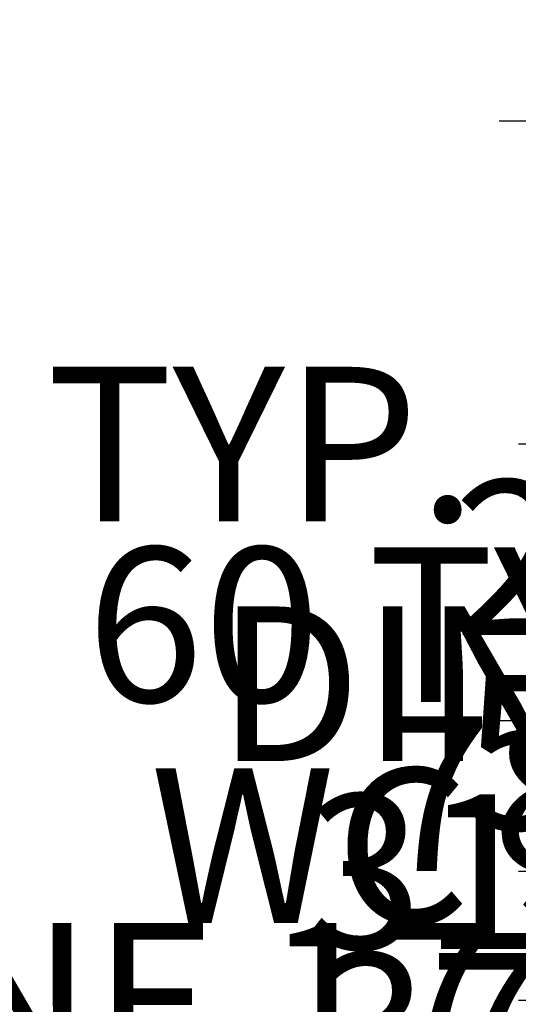
# Model space of a CAD drawing. Units: inches. Extents: x -307 to 2141, y -58 to 895.
# Tile 8 of 28: x 237 to 469, y 312 to 770. Entities that reach past the tile are written whole.
import ezdxf

# ---------------------------------------------------------------- set-up
doc = ezdxf.new("R2010")
doc.units = ezdxf.units.IN
doc.header["$MEASUREMENT"] = 0
doc.layers.add('A-ANNO-DIMS', color=2, linetype='Continuous', lineweight=18)
doc.styles.get("Standard").update_dxf_attribs({"font": 'arial.ttf'})
doc.dimstyles.get("Standard").update_dxf_attribs({"dimtxt": 72, "dimasz": 48, "dimexe": 0.18, "dimexo": 0.0625, "dimgap": 0.09, "dimtad": 0, "dimtih": 1, "dimtoh": 1, "dimdec": 0, "dimrnd": 48, "dimzin": 0, "dimdsep": 46, "dimlunit": 3, "dimtxsty": 'Standard', "dimcen": 0.09, "dimadec": 0, "dimazin": 0, "dimtfac": 1, "dimtdec": 0, "dimtofl": 0, "dimtmove": 0, "dimatfit": 3, "dimfxl": 1, "dimtolj": 1, "dimtzin": 0, "dimarcsym": 0})

# ---------------------------------------------------------------- blocks, each defined once
blk = doc.blocks.new('*D26')
at = {"layer": 'A-ANNO-DIMS', "color": 0, "lineweight": -2, "transparency": 16777216}
for p, q in [((565.34, 584.2), (565.34, 572.08)), ((645.34, 584.2), (645.34, 572.08)), ((517.34, 572.26), (469.34, 572.26)), ((693.34, 572.26), (741.34, 572.26))]:
    blk.add_line(p, q, dxfattribs=at)
at = {"layer": 'A-ANNO-DIMS', "color": 0, "transparency": 16777216}
for points in [[(517.34, 580.26), (517.34, 564.26), (565.34, 572.26)], [(693.34, 580.26), (693.34, 564.26), (645.34, 572.26)]]:
    blk.add_solid(points, dxfattribs=at)
at = {"layer": 'Defpoints', "color": 0, "transparency": 16777216}
for p in [(565.34, 584.26), (645.34, 584.26), (565.34, 572.26)]:
    blk.add_point(p, dxfattribs=at)
at = {"layer": 'A-ANNO-DIMS', "color": 0, "transparency": 16777216, "insert": (178.23, 572.26), "char_height": 72, "attachment_point": 5}
blk.add_mtext('\\A1;BED 80 TYP.', dxfattribs=at)
blk = doc.blocks.new('*D27')
at = {"layer": 'A-ANNO-DIMS', "color": 0, "lineweight": -2, "transparency": 16777216}
for p, q in [((657.34, 692.26), (657.34, 740.26)), ((645.4, 644.26), (657.52, 644.26)), ((645.4, 584.26), (657.52, 584.26)), ((657.34, 536.26), (657.34, 488.26)), ((657.34, 488.26), (609.34, 488.26))]:
    blk.add_line(p, q, dxfattribs=at)
at = {"layer": 'A-ANNO-DIMS', "color": 0, "transparency": 16777216}
for points in [[(649.34, 692.26), (665.34, 692.26), (657.34, 644.26)], [(649.34, 536.26), (665.34, 536.26), (657.34, 584.26)]]:
    blk.add_solid(points, dxfattribs=at)
at = {"layer": 'Defpoints', "color": 0, "transparency": 16777216}
for p in [(645.34, 644.26), (645.34, 584.26), (657.34, 584.26)]:
    blk.add_point(p, dxfattribs=at)
at = {"layer": 'A-ANNO-DIMS', "color": 0, "transparency": 16777216, "insert": (433.81, 488.26), "char_height": 72, "attachment_point": 5}
blk.add_mtext('\\A1;60 TYP.', dxfattribs=at)
blk = doc.blocks.new('*D28')
at = {"layer": 'A-ANNO-DIMS', "color": 0, "lineweight": -2, "transparency": 16777216}
for p, q in [((795.36, 433.55), (777.92, 433.55)), ((778.1, 385.55), (778.1, 366.07)), ((795.36, 318.07), (777.92, 318.07)), ((778.1, 318.07), (778.1, 270.07)), ((778.1, 270.07), (730.1, 270.07))]:
    blk.add_line(p, q, dxfattribs=at)
at = {"layer": 'A-ANNO-DIMS', "color": 0, "transparency": 16777216}
for points in [[(770.1, 385.55), (786.1, 385.55), (778.1, 433.55)], [(770.1, 366.07), (786.1, 366.07), (778.1, 318.07)]]:
    blk.add_solid(points, dxfattribs=at)
at = {"layer": 'Defpoints', "color": 0, "transparency": 16777216}
for p in [(795.42, 433.55), (778.1, 318.07), (795.42, 318.07)]:
    blk.add_point(p, dxfattribs=at)
at = {"layer": 'A-ANNO-DIMS', "color": 0, "transparency": 16777216, "insert": (534.42, 270.07), "char_height": 72, "attachment_point": 5}
blk.add_mtext('\\A1;BED 115', dxfattribs=at)
blk = doc.blocks.new('*D31')
at = {"layer": 'A-ANNO-DIMS', "color": 0, "lineweight": -2, "transparency": 16777216}
for p, q in [((556.34, 448.77), (556.34, 443.25)), ((565.34, 448.77), (565.34, 443.25)), ((508.34, 443.43), (460.34, 443.43)), ((613.34, 443.43), (661.34, 443.43))]:
    blk.add_line(p, q, dxfattribs=at)
at = {"layer": 'A-ANNO-DIMS', "color": 0, "transparency": 16777216}
for points in [[(508.34, 451.43), (508.34, 435.43), (556.34, 443.43)], [(613.34, 451.43), (613.34, 435.43), (565.34, 443.43)]]:
    blk.add_solid(points, dxfattribs=at)
at = {"layer": 'Defpoints', "color": 0, "transparency": 16777216}
for p in [(556.34, 448.83), (565.34, 448.83), (565.34, 443.43)]:
    blk.add_point(p, dxfattribs=at)
at = {"layer": 'A-ANNO-DIMS', "color": 0, "transparency": 16777216, "insert": (808.69, 443.43), "char_height": 72, "attachment_point": 5}
blk.add_mtext('\\A1;9 TYP.', dxfattribs=at)
blk = doc.blocks.new('*D36')
at = {"layer": 'A-ANNO-DIMS', "color": 0, "lineweight": -2, "transparency": 16777216}
for p, q in [((871.71, 562.4), (871.76, 610.4)), ((876.55, 514.4), (871.47, 514.4)), ((876.51, 481.35), (871.44, 481.36)), ((871.56, 433.36), (871.51, 385.36)), ((871.51, 385.36), (823.51, 385.36))]:
    blk.add_line(p, q, dxfattribs=at)
at = {"layer": 'A-ANNO-DIMS', "color": 0, "transparency": 16777216}
for points in [[(863.71, 562.41), (879.71, 562.4), (871.65, 514.4)], [(863.56, 433.37), (879.56, 433.35), (871.62, 481.36)]]:
    blk.add_solid(points, dxfattribs=at)
at = {"layer": 'Defpoints', "color": 0, "transparency": 16777216}
for p in [(876.61, 514.4), (871.62, 481.36), (876.57, 481.35)]:
    blk.add_point(p, dxfattribs=at)
at = {"layer": 'A-ANNO-DIMS', "color": 0, "transparency": 16777216, "insert": (548.95, 385.36), "char_height": 72, "attachment_point": 5}
blk.add_mtext('\\A1;WC 33 TYP.', dxfattribs=at)
blk = doc.blocks.new('*D37')
at = {"layer": 'A-ANNO-DIMS', "color": 0, "lineweight": -2, "transparency": 16777216}
for p, q in [((828.62, 519.41), (780.62, 519.46)), ((876.61, 514.46), (876.62, 519.54)), ((897.61, 514.44), (897.62, 519.51)), ((945.62, 519.28), (993.62, 519.22))]:
    blk.add_line(p, q, dxfattribs=at)
at = {"layer": 'A-ANNO-DIMS', "color": 0, "transparency": 16777216}
for points in [[(828.63, 527.41), (828.61, 511.41), (876.62, 519.36)], [(945.63, 527.28), (945.61, 511.28), (897.62, 519.33)]]:
    blk.add_solid(points, dxfattribs=at)
at = {"layer": 'Defpoints', "color": 0, "transparency": 16777216}
for p in [(876.62, 519.36), (876.61, 514.4), (897.61, 514.38)]:
    blk.add_point(p, dxfattribs=at)
at = {"layer": 'A-ANNO-DIMS', "color": 0, "transparency": 16777216, "insert": (604.68, 519.46), "char_height": 72, "attachment_point": 5}
blk.add_mtext('\\A1;21 TYP.', dxfattribs=at)
blk = doc.blocks.new('*D38')
at = {"layer": 'A-ANNO-DIMS', "color": 0, "lineweight": -2, "transparency": 16777216}
for p, q in [((598.5, 222.79), (550.5, 222.79)), ((646.5, 213.85), (646.5, 222.97)), ((706.5, 213.85), (706.5, 222.97)), ((754.5, 222.79), (802.5, 222.79))]:
    blk.add_line(p, q, dxfattribs=at)
at = {"layer": 'A-ANNO-DIMS', "color": 0, "transparency": 16777216}
for points in [[(598.5, 230.79), (598.5, 214.79), (646.5, 222.79)], [(754.5, 230.79), (754.5, 214.79), (706.5, 222.79)]]:
    blk.add_solid(points, dxfattribs=at)
at = {"layer": 'Defpoints', "color": 0, "transparency": 16777216}
for p in [(646.5, 222.79), (646.5, 213.79), (706.5, 213.79)]:
    blk.add_point(p, dxfattribs=at)
at = {"layer": 'A-ANNO-DIMS', "color": 0, "transparency": 16777216, "insert": (97.26, 222.79), "char_height": 72, "attachment_point": 5}
blk.add_mtext('\\A1;LOVESEAT 60 TYP.', dxfattribs=at)
blk = doc.blocks.new('*D48')
at = {"layer": 'A-ANNO-DIMS', "color": 0, "lineweight": -2, "transparency": 16777216}
for p, q in [((724, 313.98), (724, 361.98)), ((732.94, 265.98), (723.82, 265.98)), ((732.94, 205.98), (723.82, 205.98)), ((724, 157.98), (724, 109.98)), ((724, 109.98), (676, 109.98))]:
    blk.add_line(p, q, dxfattribs=at)
at = {"layer": 'A-ANNO-DIMS', "color": 0, "transparency": 16777216}
for points in [[(716, 313.98), (732, 313.98), (724, 265.98)], [(716, 157.98), (732, 157.98), (724, 205.98)]]:
    blk.add_solid(points, dxfattribs=at)
at = {"layer": 'Defpoints', "color": 0, "transparency": 16777216}
for p in [(733, 265.98), (724, 205.98), (733, 205.98)]:
    blk.add_point(p, dxfattribs=at)
at = {"layer": 'A-ANNO-DIMS', "color": 0, "transparency": 16777216, "insert": (321.56, 109.98), "char_height": 72, "attachment_point": 5}
blk.add_mtext('\\A1;MEDIA UNIT 60', dxfattribs=at)
blk = doc.blocks.new('*D50')
at = {"layer": 'A-ANNO-DIMS', "color": 0, "lineweight": -2, "transparency": 16777216}
for p, q in [((517.34, 313.33), (469.34, 313.33)), ((565.34, 315.8), (565.34, 313.15)), ((582.27, 315.8), (582.27, 313.15)), ((630.27, 313.33), (678.27, 313.33))]:
    blk.add_line(p, q, dxfattribs=at)
at = {"layer": 'A-ANNO-DIMS', "color": 0, "transparency": 16777216}
for points in [[(517.34, 321.33), (517.34, 305.33), (565.34, 313.33)], [(630.27, 321.33), (630.27, 305.33), (582.27, 313.33)]]:
    blk.add_solid(points, dxfattribs=at)
at = {"layer": 'Defpoints', "color": 0, "transparency": 16777216}
for p in [(565.34, 315.87), (565.34, 313.33), (582.27, 315.87)]:
    blk.add_point(p, dxfattribs=at)
at = {"layer": 'A-ANNO-DIMS', "color": 0, "transparency": 16777216, "insert": (226.65, 313.33), "char_height": 72, "attachment_point": 5}
blk.add_mtext('\\A1;PHONE 17', dxfattribs=at)
blk = doc.blocks.new('*D52')
at = {"layer": 'A-ANNO-DIMS', "color": 0, "lineweight": -2, "transparency": 16777216}
for p, q in [((660.21, 554.25), (660.21, 602.25)), ((673.8, 506.25), (660.03, 506.25)), ((673.8, 415.25), (660.03, 415.25)), ((660.21, 367.25), (660.21, 319.25))]:
    blk.add_line(p, q, dxfattribs=at)
at = {"layer": 'A-ANNO-DIMS', "color": 0, "transparency": 16777216}
for points in [[(652.21, 554.25), (668.21, 554.25), (660.21, 506.25)], [(652.21, 367.25), (668.21, 367.25), (660.21, 415.25)]]:
    blk.add_solid(points, dxfattribs=at)
at = {"layer": 'Defpoints', "color": 0, "transparency": 16777216}
for p in [(673.86, 506.25), (660.21, 415.25), (673.86, 415.25)]:
    blk.add_point(p, dxfattribs=at)
at = {"layer": 'A-ANNO-DIMS', "color": 0, "transparency": 16777216, "insert": (660.21, 460.75), "char_height": 72, "attachment_point": 5}
blk.add_mtext('\\A1;DINING SET 91', dxfattribs=at)
blk = doc.blocks.new('*D55')
at = {"layer": 'A-ANNO-DIMS', "color": 0, "lineweight": -2, "transparency": 16777216}
for p, q in [((517.34, 373.35), (469.34, 373.35)), ((565.34, 364.41), (565.34, 373.53)), ((596.34, 364.41), (596.34, 373.53)), ((644.34, 373.35), (692.34, 373.35))]:
    blk.add_line(p, q, dxfattribs=at)
at = {"layer": 'A-ANNO-DIMS', "color": 0, "transparency": 16777216}
for points in [[(517.34, 381.35), (517.34, 365.35), (565.34, 373.35)], [(644.34, 381.35), (644.34, 365.35), (596.34, 373.35)]]:
    blk.add_solid(points, dxfattribs=at)
at = {"layer": 'Defpoints', "color": 0, "transparency": 16777216}
for p in [(565.34, 373.35), (565.34, 364.35), (596.34, 364.35)]:
    blk.add_point(p, dxfattribs=at)
at = {"layer": 'A-ANNO-DIMS', "color": 0, "transparency": 16777216, "insert": (424.65, 373.35), "char_height": 72, "attachment_point": 5}
blk.add_mtext('\\A1;31', dxfattribs=at)
blk = doc.blocks.new('*D58')
at = {"layer": 'A-ANNO-DIMS', "color": 0, "lineweight": -2, "transparency": 16777216}
for p, q in [((624.38, 334.8), (624.38, 382.8)), ((611.84, 286.8), (624.56, 286.8)), ((611.84, 202.8), (624.56, 202.8)), ((624.38, 154.8), (624.38, 106.8))]:
    blk.add_line(p, q, dxfattribs=at)
at = {"layer": 'A-ANNO-DIMS', "color": 0, "transparency": 16777216}
for points in [[(616.38, 334.8), (632.38, 334.8), (624.38, 286.8)], [(616.38, 154.8), (632.38, 154.8), (624.38, 202.8)]]:
    blk.add_solid(points, dxfattribs=at)
at = {"layer": 'Defpoints', "color": 0, "transparency": 16777216}
for p in [(611.78, 286.8), (624.38, 286.8), (611.78, 202.8)]:
    blk.add_point(p, dxfattribs=at)
at = {"layer": 'A-ANNO-DIMS', "color": 0, "transparency": 16777216, "insert": (624.38, 244.8), "char_height": 72, "attachment_point": 5}
blk.add_mtext('\\A1;SOFA 84', dxfattribs=at)
blk = doc.blocks.new('*D59')
at = {"layer": 'A-ANNO-DIMS', "color": 0, "lineweight": -2, "transparency": 16777216}
for p, q in [((527.11, 299.4), (479.11, 299.4)), ((575.11, 286.86), (575.11, 299.58)), ((611.78, 286.86), (611.78, 299.58)), ((659.78, 299.4), (707.78, 299.4))]:
    blk.add_line(p, q, dxfattribs=at)
at = {"layer": 'A-ANNO-DIMS', "color": 0, "transparency": 16777216}
for points in [[(527.11, 307.4), (527.11, 291.4), (575.11, 299.4)], [(659.78, 307.4), (659.78, 291.4), (611.78, 299.4)]]:
    blk.add_solid(points, dxfattribs=at)
at = {"layer": 'Defpoints', "color": 0, "transparency": 16777216}
for p in [(575.11, 299.4), (575.11, 286.8), (611.78, 286.8)]:
    blk.add_point(p, dxfattribs=at)
at = {"layer": 'A-ANNO-DIMS', "color": 0, "transparency": 16777216, "insert": (427.48, 299.4), "char_height": 72, "attachment_point": 5}
blk.add_mtext('\\A1;37', dxfattribs=at)
blk = doc.blocks.new('*D64')
at = {"layer": 'A-ANNO-DIMS', "color": 0, "lineweight": -2, "transparency": 16777216}
for p, q in [((556.27, 691.34), (524.95, 691.34)), ((525.13, 643.34), (525.13, 465.69)), ((525.13, 214.34), (525.13, 391.99)), ((556.27, 166.34), (524.95, 166.34))]:
    blk.add_line(p, q, dxfattribs=at)
at = {"layer": 'A-ANNO-DIMS', "color": 0, "transparency": 16777216}
for points in [[(517.13, 643.34), (533.13, 643.34), (525.13, 691.34)], [(517.13, 214.34), (533.13, 214.34), (525.13, 166.34)]]:
    blk.add_solid(points, dxfattribs=at)
at = {"layer": 'Defpoints', "color": 0, "transparency": 16777216}
for p in [(525.13, 691.34), (556.34, 691.34), (556.34, 166.34)]:
    blk.add_point(p, dxfattribs=at)
at = {"layer": 'A-ANNO-DIMS', "color": 0, "transparency": 16777216, "insert": (525.13, 428.84), "char_height": 72, "attachment_point": 5}
blk.add_mtext('\\A1;525', dxfattribs=at)
blk = doc.blocks.new('*D66')
at = {"layer": 'A-ANNO-DIMS', "color": 0, "lineweight": -2, "transparency": 16777216}
for p, q in [((525.13, 382.34), (525.13, 430.34)), ((556.27, 334.34), (524.95, 334.34)), ((565.27, 304.34), (524.95, 304.34)), ((525.13, 256.34), (525.13, 208.34)), ((525.13, 208.34), (477.13, 208.34))]:
    blk.add_line(p, q, dxfattribs=at)
at = {"layer": 'A-ANNO-DIMS', "color": 0, "transparency": 16777216}
for points in [[(517.13, 382.34), (533.13, 382.34), (525.13, 334.34)], [(517.13, 256.34), (533.13, 256.34), (525.13, 304.34)]]:
    blk.add_solid(points, dxfattribs=at)
at = {"layer": 'Defpoints', "color": 0, "transparency": 16777216}
for p in [(556.34, 334.34), (525.13, 304.34), (565.34, 304.34)]:
    blk.add_point(p, dxfattribs=at)
at = {"layer": 'A-ANNO-DIMS', "color": 0, "transparency": 16777216, "insert": (425.62, 208.34), "char_height": 72, "attachment_point": 5}
blk.add_mtext('\\A1;30', dxfattribs=at)
blk = doc.blocks.new('*D67')
at = {"layer": 'A-ANNO-DIMS', "color": 0, "lineweight": -2, "transparency": 16777216}
for p, q in [((525.13, 496.83), (525.13, 544.83)), ((556.27, 448.83), (524.95, 448.83)), ((556.27, 370.34), (524.95, 370.34)), ((525.13, 322.34), (525.13, 274.34))]:
    blk.add_line(p, q, dxfattribs=at)
at = {"layer": 'A-ANNO-DIMS', "color": 0, "transparency": 16777216}
for points in [[(517.13, 496.83), (533.13, 496.83), (525.13, 448.83)], [(517.13, 322.34), (533.13, 322.34), (525.13, 370.34)]]:
    blk.add_solid(points, dxfattribs=at)
at = {"layer": 'Defpoints', "color": 0, "transparency": 16777216}
for p in [(525.13, 448.83), (556.34, 448.83), (556.34, 370.34)]:
    blk.add_point(p, dxfattribs=at)
at = {"layer": 'A-ANNO-DIMS', "color": 0, "transparency": 16777216, "insert": (525.13, 409.59), "char_height": 72, "attachment_point": 5}
blk.add_mtext('\\A1;78.49', dxfattribs=at)
blk = doc.blocks.new('*D101')
at = {"layer": 'A-ANNO-DIMS', "color": 0, "lineweight": -2, "transparency": 16777216}
for p, q in [((508.34, 722.54), (460.34, 722.54)), ((556.34, 691.4), (556.34, 722.72)), ((589.36, 691.4), (589.36, 722.72)), ((637.36, 722.54), (685.36, 722.54))]:
    blk.add_line(p, q, dxfattribs=at)
at = {"layer": 'A-ANNO-DIMS', "color": 0, "transparency": 16777216}
for points in [[(508.34, 730.54), (508.34, 714.54), (556.34, 722.54)], [(637.36, 730.54), (637.36, 714.54), (589.36, 722.54)]]:
    blk.add_solid(points, dxfattribs=at)
at = {"layer": 'Defpoints', "color": 0, "transparency": 16777216}
for p in [(589.36, 722.54), (556.34, 691.34), (589.36, 691.34)]:
    blk.add_point(p, dxfattribs=at)
at = {"layer": 'A-ANNO-DIMS', "color": 0, "transparency": 16777216, "insert": (806.54, 722.54), "char_height": 72, "attachment_point": 5}
blk.add_mtext('\\A1;33.02', dxfattribs=at)

msp = doc.modelspace()

# ---------------------------------------------------------------- dimensions: what is measured, and where the dimension line sits
at = {"layer": 'A-ANNO-DIMS'}
dim = msp.add_linear_dim(base=(589.3579, 722.5448), p1=(556.3358, 691.3408), p2=(589.3579, 691.3408), dimstyle='Standard', override={"dimdec": 2, "dimlfac": 1, "dimrnd": 0, "dimzin": 0, "dimdsep": 46, "dimlunit": 2}, dxfattribs=at)
dim.commit()
dim.dimension.update_dxf_attribs({"geometry": '*D101', "text_midpoint": (806.5366, 722.5448)})
for base, p1, p2, angle, text, picture, middle in [((565.3358, 572.2648), (645.3359, 584.2648), (565.3358, 584.2648), 180, 'BED <> TYP.', '*D26', (178.2254, 572.2648)), ((657.3359, 584.2648), (645.3359, 644.2648), (645.3359, 584.2648), 270, '<> TYP.', '*D27', (433.8134, 488.2648)), ((660.2083, 415.2485), (673.8583, 506.2485), (673.8583, 415.2485), 270, 'DINING SET <>', '*D52', (660.2083, 460.7485)), ((876.6162, 519.3557), (897.6106, 514.3753), (876.6106, 514.3988), 179.935892, '<> TYP.', '*D37', (604.6763, 519.4631)), ((871.6167, 481.3581), (876.6106, 514.3988), (876.5736, 481.3526), 269.935892, 'WC <> TYP.', '*D36', (548.95, 385.3582)), ((778.0993, 318.073), (795.4208, 433.5496), (795.4208, 318.073), 270, 'BED <>', '*D28', (534.4158, 270.073)), ((565.3358, 313.3263), (582.2714, 315.8666), (565.3358, 315.8666), 180, 'PHONE <>', '*D50', (226.651, 313.3263)), ((646.4965, 222.7908), (706.4965, 213.7908), (646.4965, 213.7908), 180, 'LOVESEAT <> TYP.', '*D38', (97.2632, 222.7908)), ((624.377, 286.7976), (611.777, 202.7976), (611.777, 286.7976), 90, 'SOFA <>', '*D58', (624.377, 244.7976)), ((724.0025, 205.9815), (733.0025, 265.9815), (733.0025, 205.9815), 270, 'MEDIA UNIT <>', '*D48', (321.5605, 109.9815))]:
    dim = msp.add_linear_dim(base=base, p1=p1, p2=p2, angle=angle, text=text, dimstyle='Standard', override={"dimdec": 0, "dimlfac": 1, "dimrnd": 0, "dimzin": 0, "dimdsep": 46, "dimlunit": 2}, dxfattribs=at)
    dim.commit()
    dim.dimension.update_dxf_attribs({"geometry": picture, "text_midpoint": middle})
for base, p1, p2, angle, override, picture, middle in [((525.1318, 691.3408), (556.3358, 166.3408), (556.3358, 691.3408), 90, {"dimdec": 0, "dimlfac": 1, "dimrnd": 0, "dimzin": 0, "dimdsep": 46, "dimlunit": 2}, '*D64', (525.1318, 428.8408)), ((525.1318, 448.8333), (556.3358, 370.3416), (556.3358, 448.8333), 90, {"dimdec": 2, "dimlfac": 1, "dimrnd": 0, "dimzin": 0, "dimdsep": 46, "dimlunit": 2}, '*D67', (525.1318, 409.5874)), ((525.1318, 304.3408), (556.3358, 334.3416), (565.3358, 304.3408), 90, {"dimdec": 0, "dimlfac": 1, "dimrnd": 0, "dimzin": 0, "dimdsep": 46, "dimlunit": 2}, '*D66', (425.6203, 208.3408)), ((565.3358, 373.3488), (596.3358, 364.3488), (565.3358, 364.3488), 180, {"dimdec": 0, "dimlfac": 1, "dimrnd": 0, "dimzin": 0, "dimdsep": 46, "dimlunit": 2}, '*D55', (424.651, 373.3488)), ((575.1104, 299.3976), (611.777, 286.7976), (575.1104, 286.7976), 180, {"dimdec": 0, "dimlfac": 1, "dimrnd": 0, "dimzin": 0, "dimdsep": 46, "dimlunit": 2}, '*D59', (427.476, 299.3976))]:
    dim = msp.add_linear_dim(base=base, p1=p1, p2=p2, angle=angle, dimstyle='Standard', override=override, dxfattribs=at)
    dim.commit()
    dim.dimension.update_dxf_attribs({"geometry": picture, "text_midpoint": middle})
dim = msp.add_linear_dim(base=(565.3358, 443.4333), p1=(556.3358, 448.8333), p2=(565.3358, 448.8333), text='<> TYP.', dimstyle='Standard', override={"dimdec": 0, "dimlfac": 1, "dimrnd": 0, "dimzin": 0, "dimdsep": 46, "dimlunit": 2}, dxfattribs=at)
dim.commit()
dim.dimension.update_dxf_attribs({"geometry": '*D31', "text_midpoint": (808.6919, 443.4333)})

doc.saveas('drawing.dxf')
